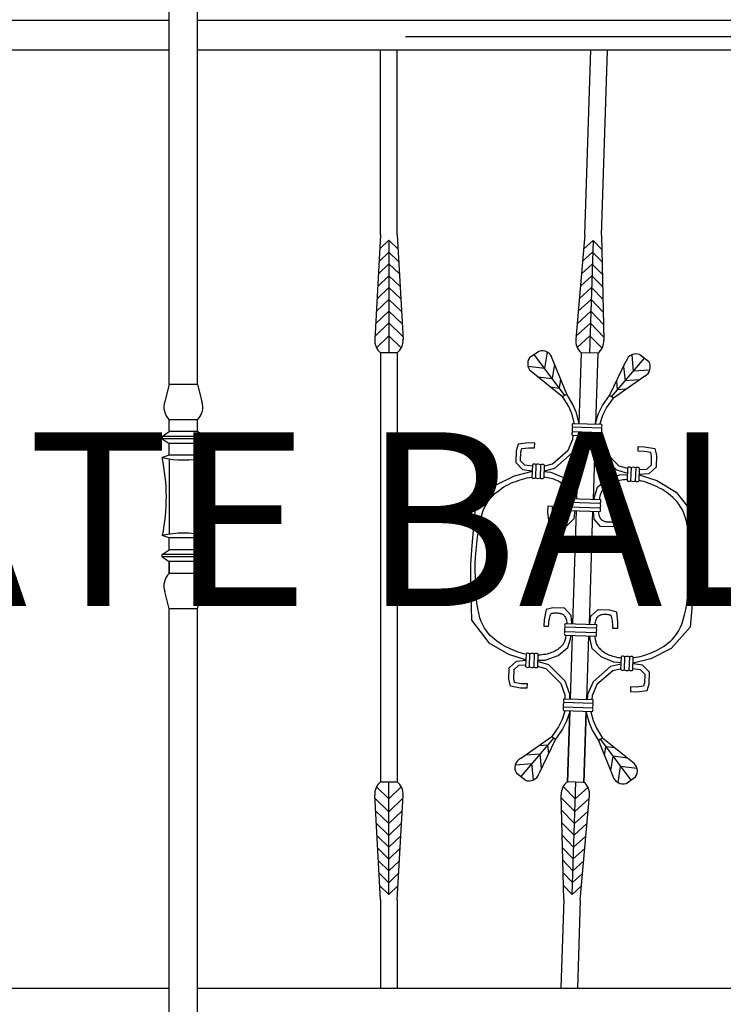
# Model space of a CAD drawing. Units: inches. Extents: x 2278 to 7495, y -71 to 1198.
# Tile 23 of 44: x 5060 to 5084, y 126 to 160. Entities that reach past the tile are written whole.
import ezdxf

# ---------------------------------------------------------------- set-up
doc = ezdxf.new("R2010")
doc.units = ezdxf.units.IN
doc.header["$MEASUREMENT"] = 0
doc.layers.add('A-ANNO-DIMS', color=2, linetype='Continuous', lineweight=18)
doc.layers.add('A-ELEV', color=7, linetype='Continuous', lineweight=25)
doc.styles.get("Standard").update_dxf_attribs({"font": 'arial.ttf'})
doc.dimstyles.get("Standard").update_dxf_attribs({"dimtxt": 6, "dimasz": 3, "dimexe": 0.18, "dimexo": 0.0625, "dimgap": 0.09, "dimtad": 0, "dimtih": 1, "dimtoh": 1, "dimdec": 0, "dimzin": 0, "dimdsep": 46, "dimlunit": 3, "dimtxsty": 'Standard', "dimblk": 'ARCHTICK', "dimcen": 0.09, "dimadec": 0, "dimazin": 0, "dimtfac": 1, "dimtdec": 0, "dimtofl": 0, "dimtmove": 0, "dimatfit": 3, "dimfxl": 1, "dimtolj": 1, "dimtzin": 0, "dimarcsym": 0})

# ---------------------------------------------------------------- blocks, each defined once
blk = doc.blocks.new('BALUSTER-ORNATE-A')
for p, q in [((3.585, 26.003), (3.585, 32.384)), ((4.155, 26.003), (4.155, 32.38)), ((3.585, 26.003), (3.383, 22.393)), ((4.155, 26.003), (4.357, 22.393)), ((3.558, 25.516), (3.87, 25.818)), ((3.87, 25.818), (3.87, 21.929)), ((4.182, 25.516), (3.87, 25.818)), ((3.533, 25.084), (3.87, 25.41)), ((4.207, 25.084), (3.87, 25.41)), ((3.509, 24.653), (3.87, 25.001)), ((4.231, 24.653), (3.87, 25.001)), ((3.485, 24.221), (3.87, 24.593)), ((4.255, 24.221), (3.87, 24.593)), ((3.461, 23.79), (3.87, 24.185)), ((4.279, 23.79), (3.87, 24.185)), ((3.437, 23.358), (3.87, 23.777)), ((4.303, 23.358), (3.87, 23.777)), ((3.413, 22.927), (3.87, 23.369)), ((4.327, 22.927), (3.87, 23.369)), ((3.388, 22.495), (3.87, 22.961)), ((4.352, 22.495), (3.87, 22.961)), ((3.442, 22.106), (3.87, 22.52)), ((4.299, 22.106), (3.87, 22.52)), ((2.128, 21.929), (1.813, 21.699)), ((3.063, 20.442), (1.97, 21.814)), ((2.412, 21.914), (2.339, 21.352)), ((3.585, 21.929), (3.585, 19.485)), ((4.155, 21.929), (3.585, 21.929)), ((4.155, 21.929), (4.155, 19.485)), ((4.677, 20.442), (5.77, 21.814)), ((5.328, 21.914), (5.401, 21.352)), ((5.612, 21.929), (5.927, 21.699)), ((1.774, 21.406), (2.339, 21.352)), ((3.131, 20.487), (2.594, 21.696)), ((2.678, 21.507), (2.613, 21.007)), ((4.609, 20.487), (5.146, 21.696)), ((5.062, 21.507), (5.127, 21.007)), ((5.966, 21.406), (5.401, 21.352)), ((1.936, 21.192), (2.995, 20.398)), ((5.804, 21.192), (4.745, 20.398)), ((2.111, 21.055), (2.613, 21.007)), ((2.907, 20.992), (2.868, 20.688)), ((4.833, 20.992), (4.872, 20.688)), ((5.629, 21.055), (5.127, 21.007)), ((2.562, 20.717), (2.868, 20.688)), ((2.995, 20.398), (3.131, 20.487)), ((3.217, 20.057), (2.995, 20.398)), ((3.36, 20.135), (3.131, 20.487)), ((4.38, 20.135), (4.609, 20.487)), ((4.523, 20.057), (4.745, 20.398)), ((4.745, 20.398), (4.609, 20.487)), ((5.178, 20.717), (4.872, 20.688)), ((3.337, 19.795), (3.217, 20.057)), ((3.49, 19.852), (3.36, 20.135)), ((4.25, 19.852), (4.38, 20.135)), ((4.403, 19.795), (4.523, 20.057)), ((3.421, 19.506), (3.337, 19.795)), ((3.585, 19.526), (3.49, 19.852)), ((4.155, 19.526), (4.25, 19.852)), ((4.319, 19.506), (4.403, 19.795)), ((3.37, 19.485), (4.37, 19.485)), ((3.42, 19.485), (3.421, 19.506)), ((3.583, 19.485), (3.585, 19.526)), ((4.157, 19.485), (4.155, 19.526)), ((4.32, 19.485), (4.319, 19.506)), ((3.37, 19.363), (4.37, 19.363)), ((3.37, 19.2), (4.37, 19.2)), ((3.37, 19.077), (4.37, 19.077)), ((3.396, 18.942), (3.402, 19.077)), ((3.558, 18.908), (3.565, 19.077)), ((3.585, 19.077), (3.585, 16.887)), ((4.155, 19.077), (4.155, 16.887)), ((4.182, 18.908), (4.175, 19.077)), ((4.344, 18.942), (4.338, 19.077)), ((1.513, 18.705), (1.449, 18.469)), ((1.866, 18.759), (1.513, 18.705)), ((2.084, 18.759), (1.866, 18.759)), ((2.084, 18.596), (2.084, 18.759)), ((3.247, 18.557), (3.396, 18.942)), ((3.385, 18.463), (3.558, 18.908)), ((4.355, 18.463), (4.182, 18.908)), ((4.493, 18.557), (4.344, 18.942)), ((5.656, 18.596), (5.656, 18.759)), ((5.656, 18.759), (5.874, 18.759)), ((5.874, 18.759), (6.227, 18.705)), ((6.227, 18.705), (6.291, 18.469)), ((1.449, 18.469), (1.449, 18.069)), ((1.612, 18.447), (1.642, 18.56)), ((1.612, 18.138), (1.612, 18.447)), ((1.642, 18.56), (1.879, 18.596)), ((1.879, 18.596), (2.084, 18.596)), ((2.719, 18.062), (3.247, 18.557)), ((2.801, 17.915), (3.385, 18.463)), ((4.939, 17.915), (4.355, 18.463)), ((5.021, 18.062), (4.493, 18.557)), ((5.861, 18.596), (5.656, 18.596)), ((6.098, 18.56), (5.861, 18.596)), ((6.128, 18.447), (6.098, 18.56)), ((6.128, 18.138), (6.128, 18.447)), ((6.291, 18.469), (6.291, 18.069)), ((1.449, 18.069), (1.694, 17.833)), ((1.767, 17.989), (1.612, 18.138)), ((2.026, 18.021), (2.026, 17.565)), ((2.148, 18.021), (2.148, 17.565)), ((2.311, 18.021), (2.311, 17.565)), ((2.434, 18.021), (2.434, 17.565)), ((2.462, 17.993), (2.719, 18.062)), ((5.278, 17.993), (5.021, 18.062)), ((5.306, 18.021), (5.306, 17.565)), ((5.429, 18.021), (5.429, 17.565)), ((5.592, 18.021), (5.592, 17.565)), ((5.714, 18.021), (5.714, 17.565)), ((5.973, 17.989), (6.128, 18.138)), ((6.291, 18.069), (6.046, 17.833)), ((2.026, 17.782), (1.412, 17.603)), ((1.694, 17.833), (2.026, 17.797)), ((2.026, 17.961), (1.767, 17.989)), ((2.434, 17.99), (2.462, 17.993)), ((2.434, 17.826), (2.492, 17.833)), ((2.683, 17.766), (2.434, 17.777)), ((2.492, 17.833), (2.801, 17.915)), ((3.128, 17.594), (2.683, 17.766)), ((4.612, 17.594), (5.057, 17.766)), ((5.248, 17.833), (4.939, 17.915)), ((5.057, 17.766), (5.306, 17.777)), ((5.306, 17.826), (5.248, 17.833)), ((5.306, 17.99), (5.278, 17.993)), ((5.714, 17.961), (5.973, 17.989)), ((6.046, 17.833), (5.714, 17.797)), ((5.714, 17.782), (6.328, 17.603)), ((1.412, 17.603), (0.722, 17.231)), ((1.23, 17.309), (1.309, 17.35)), ((1.309, 17.35), (1.389, 17.388)), ((1.389, 17.388), (1.469, 17.422)), ((1.469, 17.422), (1.549, 17.454)), ((1.549, 17.454), (1.627, 17.484)), ((1.627, 17.484), (1.705, 17.51)), ((1.705, 17.51), (1.782, 17.533)), ((1.782, 17.533), (1.858, 17.553)), ((1.858, 17.553), (1.933, 17.571)), ((1.933, 17.571), (2.007, 17.585)), ((2.007, 17.585), (2.026, 17.587)), ((2.434, 17.606), (2.499, 17.6)), ((2.499, 17.6), (2.563, 17.592)), ((2.563, 17.592), (2.624, 17.582)), ((2.624, 17.582), (2.683, 17.57)), ((2.683, 17.57), (2.739, 17.556)), ((2.739, 17.556), (2.792, 17.54)), ((2.792, 17.54), (2.843, 17.522)), ((2.843, 17.522), (2.891, 17.503)), ((2.891, 17.503), (2.937, 17.482)), ((2.937, 17.482), (2.981, 17.46)), ((2.981, 17.46), (3.024, 17.436)), ((3.024, 17.436), (3.064, 17.41)), ((3.064, 17.41), (3.102, 17.384)), ((3.102, 17.384), (3.138, 17.357)), ((3.446, 17.313), (3.128, 17.594)), ((3.138, 17.357), (3.171, 17.329)), ((3.171, 17.329), (3.201, 17.301)), ((4.294, 17.313), (4.612, 17.594)), ((4.569, 17.329), (4.539, 17.301)), ((4.602, 17.357), (4.569, 17.329)), ((4.638, 17.384), (4.602, 17.357)), ((4.676, 17.41), (4.638, 17.384)), ((4.716, 17.436), (4.676, 17.41)), ((4.759, 17.46), (4.716, 17.436)), ((4.803, 17.482), (4.759, 17.46)), ((4.849, 17.503), (4.803, 17.482)), ((4.897, 17.522), (4.849, 17.503)), ((4.948, 17.54), (4.897, 17.522)), ((5.001, 17.556), (4.948, 17.54)), ((5.057, 17.57), (5.001, 17.556)), ((5.116, 17.582), (5.057, 17.57)), ((5.177, 17.592), (5.116, 17.582)), ((5.241, 17.6), (5.177, 17.592)), ((5.306, 17.606), (5.241, 17.6)), ((5.733, 17.585), (5.714, 17.587)), ((5.807, 17.571), (5.733, 17.585)), ((5.882, 17.553), (5.807, 17.571)), ((5.958, 17.533), (5.882, 17.553)), ((6.035, 17.51), (5.958, 17.533)), ((6.113, 17.484), (6.035, 17.51)), ((6.191, 17.454), (6.113, 17.484)), ((6.271, 17.422), (6.191, 17.454)), ((6.351, 17.388), (6.271, 17.422)), ((6.328, 17.603), (7.018, 17.231)), ((6.431, 17.35), (6.351, 17.388)), ((6.51, 17.309), (6.431, 17.35)), ((0.722, 17.231), (0.096, 16.469)), ((0.764, 16.975), (0.839, 17.043)), ((0.839, 17.043), (0.916, 17.105)), ((0.916, 17.105), (0.993, 17.163)), ((0.993, 17.163), (1.071, 17.216)), ((1.071, 17.216), (1.15, 17.265)), ((1.15, 17.265), (1.23, 17.309)), ((3.201, 17.301), (3.228, 17.272)), ((3.228, 17.272), (3.252, 17.244)), ((3.252, 17.244), (3.272, 17.217)), ((3.272, 17.217), (3.288, 17.19)), ((3.288, 17.19), (3.303, 17.162)), ((3.303, 17.162), (3.316, 17.134)), ((3.316, 17.134), (3.327, 17.104)), ((3.327, 17.104), (3.337, 17.072)), ((3.337, 17.072), (3.346, 17.038)), ((3.346, 17.038), (3.354, 17.001)), ((3.354, 17.001), (3.361, 16.962)), ((3.528, 17.004), (3.446, 17.313)), ((3.542, 16.887), (3.528, 17.004)), ((4.198, 16.887), (4.212, 17.004)), ((4.212, 17.004), (4.294, 17.313)), ((4.386, 17.001), (4.379, 16.962)), ((4.394, 17.038), (4.386, 17.001)), ((4.403, 17.072), (4.394, 17.038)), ((4.413, 17.104), (4.403, 17.072)), ((4.424, 17.134), (4.413, 17.104)), ((4.437, 17.162), (4.424, 17.134)), ((4.452, 17.19), (4.437, 17.162)), ((4.468, 17.217), (4.452, 17.19)), ((4.489, 17.244), (4.468, 17.217)), ((4.512, 17.272), (4.489, 17.244)), ((4.539, 17.301), (4.512, 17.272)), ((6.59, 17.265), (6.51, 17.309)), ((6.669, 17.216), (6.59, 17.265)), ((6.747, 17.163), (6.669, 17.216)), ((6.824, 17.105), (6.747, 17.163)), ((6.901, 17.043), (6.824, 17.105)), ((6.976, 16.975), (6.901, 17.043)), ((7.018, 17.231), (7.644, 16.469)), ((0.495, 16.624), (0.557, 16.727)), ((0.557, 16.727), (0.623, 16.819)), ((0.623, 16.819), (0.692, 16.9)), ((0.692, 16.9), (0.764, 16.975)), ((3.329, 16.887), (4.411, 16.887)), ((3.329, 16.764), (4.411, 16.764)), ((3.361, 16.962), (3.368, 16.922)), ((3.368, 16.922), (3.374, 16.887)), ((4.372, 16.922), (4.366, 16.887)), ((4.379, 16.962), (4.372, 16.922)), ((7.048, 16.9), (6.976, 16.975)), ((7.117, 16.819), (7.048, 16.9)), ((7.183, 16.727), (7.117, 16.819)), ((7.245, 16.624), (7.183, 16.727)), ((0.096, 16.469), (0.025, 15.162)), ((0.34, 16.227), (0.386, 16.376)), ((0.386, 16.376), (0.438, 16.508)), ((0.438, 16.508), (0.495, 16.624)), ((2.764, 16.599), (2.602, 16.596)), ((2.602, 16.596), (2.602, 16.378)), ((2.602, 16.378), (2.656, 16.024)), ((2.766, 16.522), (2.764, 16.599)), ((2.769, 16.452), (2.766, 16.522)), ((2.775, 16.388), (2.769, 16.452)), ((2.783, 16.331), (2.775, 16.388)), ((2.792, 16.28), (2.783, 16.331)), ((3.329, 16.601), (4.411, 16.601)), ((3.329, 16.479), (4.411, 16.479)), ((3.357, 16.329), (3.346, 16.299)), ((3.368, 16.364), (3.357, 16.329)), ((3.376, 16.401), (3.368, 16.364)), ((3.383, 16.441), (3.376, 16.401)), ((3.388, 16.479), (3.383, 16.441)), ((3.528, 16.206), (3.557, 16.479)), ((3.585, 16.479), (3.585, 12.578)), ((4.155, 16.479), (4.155, 12.578)), ((4.212, 16.206), (4.183, 16.479)), ((4.352, 16.479), (4.357, 16.441)), ((4.357, 16.441), (4.364, 16.401)), ((4.364, 16.401), (4.372, 16.364)), ((4.372, 16.364), (4.383, 16.329)), ((4.383, 16.329), (4.394, 16.299)), ((4.948, 16.28), (4.957, 16.331)), ((4.957, 16.331), (4.965, 16.388)), ((4.965, 16.388), (4.971, 16.452)), ((4.971, 16.452), (4.974, 16.522)), ((4.974, 16.522), (4.976, 16.599)), ((4.976, 16.599), (5.138, 16.596)), ((5.138, 16.378), (5.084, 16.024)), ((5.138, 16.596), (5.138, 16.378)), ((7.302, 16.508), (7.245, 16.624)), ((7.354, 16.376), (7.302, 16.508)), ((7.4, 16.227), (7.354, 16.376)), ((7.644, 16.469), (7.715, 15.162)), ((0.267, 15.87), (0.3, 16.057)), ((0.3, 16.057), (0.34, 16.227)), ((2.656, 16.024), (2.892, 15.961)), ((2.803, 16.237), (2.792, 16.28)), ((2.815, 16.203), (2.803, 16.237)), ((2.825, 16.18), (2.815, 16.203)), ((2.834, 16.166), (2.825, 16.18)), ((2.84, 16.159), (2.834, 16.166)), ((2.846, 16.154), (2.84, 16.159)), ((2.852, 16.151), (2.846, 16.154)), ((2.863, 16.146), (2.852, 16.151)), ((2.88, 16.142), (2.863, 16.146)), ((2.905, 16.137), (2.88, 16.142)), ((2.936, 16.134), (2.905, 16.137)), ((2.971, 16.131), (2.936, 16.134)), ((3.008, 16.129), (2.971, 16.131)), ((3.045, 16.129), (3.008, 16.129)), ((3.081, 16.13), (3.045, 16.129)), ((3.117, 16.133), (3.081, 16.13)), ((3.15, 16.138), (3.117, 16.133)), ((3.179, 16.145), (3.15, 16.138)), ((3.205, 16.154), (3.179, 16.145)), ((3.228, 16.164), (3.205, 16.154)), ((3.249, 16.176), (3.228, 16.164)), ((3.268, 16.19), (3.249, 16.176)), ((3.286, 16.207), (3.268, 16.19)), ((3.303, 16.225), (3.286, 16.207)), ((3.292, 15.961), (3.528, 16.206)), ((3.318, 16.247), (3.303, 16.225)), ((3.333, 16.271), (3.318, 16.247)), ((3.346, 16.299), (3.333, 16.271)), ((4.448, 15.961), (4.212, 16.206)), ((4.394, 16.299), (4.407, 16.271)), ((4.407, 16.271), (4.422, 16.247)), ((4.422, 16.247), (4.437, 16.225)), ((4.437, 16.225), (4.454, 16.207)), ((4.454, 16.207), (4.472, 16.19)), ((4.472, 16.19), (4.491, 16.176)), ((4.491, 16.176), (4.512, 16.164)), ((4.512, 16.164), (4.535, 16.154)), ((4.535, 16.154), (4.561, 16.145)), ((4.561, 16.145), (4.59, 16.138)), ((4.59, 16.138), (4.623, 16.133)), ((4.623, 16.133), (4.659, 16.13)), ((4.659, 16.13), (4.695, 16.129)), ((4.695, 16.129), (4.732, 16.129)), ((4.732, 16.129), (4.769, 16.131)), ((4.769, 16.131), (4.804, 16.134)), ((4.804, 16.134), (4.835, 16.137)), ((4.835, 16.137), (4.86, 16.142)), ((5.084, 16.024), (4.848, 15.961)), ((4.86, 16.142), (4.877, 16.146)), ((4.877, 16.146), (4.888, 16.151)), ((4.888, 16.151), (4.895, 16.154)), ((4.895, 16.154), (4.9, 16.159)), ((4.9, 16.159), (4.906, 16.166)), ((4.906, 16.166), (4.915, 16.18)), ((4.915, 16.18), (4.925, 16.203)), ((4.925, 16.203), (4.937, 16.237)), ((4.937, 16.237), (4.948, 16.28)), ((7.44, 16.057), (7.4, 16.227)), ((7.473, 15.87), (7.44, 16.057)), ((0.217, 15.452), (0.239, 15.667)), ((0.239, 15.667), (0.267, 15.87)), ((2.892, 15.961), (3.292, 15.961)), ((4.848, 15.961), (4.448, 15.961)), ((7.501, 15.667), (7.473, 15.87)), ((7.523, 15.452), (7.501, 15.667)), ((0.199, 15.227), (0.217, 15.452)), ((7.541, 15.227), (7.523, 15.452)), ((0.025, 15.162), (0, 14.529)), ((0.173, 14.759), (0.185, 14.995)), ((0.185, 14.995), (0.199, 15.227)), ((7.555, 14.995), (7.541, 15.227)), ((7.567, 14.759), (7.555, 14.995)), ((7.715, 15.162), (7.74, 14.529)), ((0.163, 14.522), (0.173, 14.759)), ((7.577, 14.522), (7.567, 14.759)), ((0, 14.529), (0.025, 13.895)), ((0.173, 14.298), (0.163, 14.536)), ((0.185, 14.062), (0.173, 14.298)), ((7.555, 14.062), (7.567, 14.298)), ((7.567, 14.298), (7.577, 14.536)), ((7.74, 14.529), (7.715, 13.895)), ((0.199, 13.831), (0.185, 14.062)), ((7.541, 13.831), (7.555, 14.062)), ((0.025, 13.895), (0.096, 12.589)), ((0.217, 13.606), (0.199, 13.831)), ((0.239, 13.391), (0.217, 13.606)), ((7.501, 13.391), (7.523, 13.606)), ((7.523, 13.606), (7.541, 13.831)), ((7.715, 13.895), (7.644, 12.589)), ((0.267, 13.188), (0.239, 13.391)), ((7.473, 13.188), (7.501, 13.391)), ((0.3, 13), (0.267, 13.188)), ((0.34, 12.831), (0.3, 13)), ((2.656, 13.033), (2.602, 12.679)), ((2.892, 13.097), (2.656, 13.033)), ((2.852, 12.907), (2.863, 12.911)), ((2.863, 12.911), (2.88, 12.916)), ((2.88, 12.916), (2.905, 12.92)), ((3.292, 13.097), (2.892, 13.097)), ((2.905, 12.92), (2.936, 12.924)), ((2.936, 12.924), (2.971, 12.927)), ((2.971, 12.927), (3.008, 12.929)), ((3.008, 12.929), (3.045, 12.929)), ((3.045, 12.929), (3.081, 12.928)), ((3.081, 12.928), (3.117, 12.924)), ((3.117, 12.924), (3.15, 12.919)), ((3.15, 12.919), (3.179, 12.912)), ((3.179, 12.912), (3.205, 12.904)), ((3.528, 12.852), (3.292, 13.097)), ((4.212, 12.852), (4.448, 13.097)), ((4.448, 13.097), (4.848, 13.097)), ((4.561, 12.912), (4.535, 12.904)), ((4.59, 12.919), (4.561, 12.912)), ((4.623, 12.924), (4.59, 12.919)), ((4.659, 12.928), (4.623, 12.924)), ((4.695, 12.929), (4.659, 12.928)), ((4.732, 12.929), (4.695, 12.929)), ((4.769, 12.927), (4.732, 12.929)), ((4.804, 12.924), (4.769, 12.927)), ((4.835, 12.92), (4.804, 12.924)), ((4.86, 12.916), (4.835, 12.92)), ((4.848, 13.097), (5.084, 13.033)), ((4.877, 12.911), (4.86, 12.916)), ((4.888, 12.907), (4.877, 12.911)), ((5.084, 13.033), (5.138, 12.679)), ((7.4, 12.831), (7.44, 13)), ((7.44, 13), (7.473, 13.188)), ((0.096, 12.589), (0.722, 11.827)), ((0.386, 12.681), (0.34, 12.831)), ((0.438, 12.549), (0.386, 12.681)), ((2.602, 12.679), (2.602, 12.462)), ((2.766, 12.536), (2.769, 12.605)), ((2.769, 12.605), (2.775, 12.669)), ((2.775, 12.669), (2.783, 12.727)), ((2.783, 12.727), (2.792, 12.778)), ((2.792, 12.778), (2.803, 12.82)), ((2.803, 12.82), (2.815, 12.854)), ((2.815, 12.854), (2.825, 12.878)), ((2.825, 12.878), (2.834, 12.892)), ((2.834, 12.892), (2.84, 12.899)), ((2.84, 12.899), (2.846, 12.903)), ((2.846, 12.903), (2.852, 12.907)), ((3.205, 12.904), (3.228, 12.893)), ((3.228, 12.893), (3.249, 12.881)), ((3.249, 12.881), (3.268, 12.867)), ((3.268, 12.867), (3.286, 12.851)), ((3.286, 12.851), (3.303, 12.832)), ((3.303, 12.832), (3.318, 12.811)), ((3.318, 12.811), (3.333, 12.786)), ((3.329, 12.578), (4.411, 12.578)), ((3.333, 12.786), (3.346, 12.759)), ((3.346, 12.759), (3.357, 12.728)), ((3.357, 12.728), (3.368, 12.694)), ((3.368, 12.694), (3.376, 12.656)), ((3.376, 12.656), (3.383, 12.616)), ((3.383, 12.616), (3.388, 12.578)), ((3.557, 12.578), (3.528, 12.852)), ((4.183, 12.578), (4.212, 12.852)), ((4.357, 12.616), (4.352, 12.578)), ((4.364, 12.656), (4.357, 12.616)), ((4.372, 12.694), (4.364, 12.656)), ((4.383, 12.728), (4.372, 12.694)), ((4.394, 12.759), (4.383, 12.728)), ((4.407, 12.786), (4.394, 12.759)), ((4.422, 12.811), (4.407, 12.786)), ((4.437, 12.832), (4.422, 12.811)), ((4.454, 12.851), (4.437, 12.832)), ((4.472, 12.867), (4.454, 12.851)), ((4.491, 12.881), (4.472, 12.867)), ((4.512, 12.893), (4.491, 12.881)), ((4.535, 12.904), (4.512, 12.893)), ((4.895, 12.903), (4.888, 12.907)), ((4.9, 12.899), (4.895, 12.903)), ((4.906, 12.892), (4.9, 12.899)), ((4.915, 12.878), (4.906, 12.892)), ((4.925, 12.854), (4.915, 12.878)), ((4.937, 12.82), (4.925, 12.854)), ((4.948, 12.778), (4.937, 12.82)), ((4.957, 12.727), (4.948, 12.778)), ((4.965, 12.669), (4.957, 12.727)), ((4.971, 12.605), (4.965, 12.669)), ((4.974, 12.536), (4.971, 12.605)), ((5.138, 12.679), (5.138, 12.462)), ((7.644, 12.589), (7.018, 11.827)), ((7.302, 12.549), (7.354, 12.681)), ((7.354, 12.681), (7.4, 12.831)), ((0.495, 12.433), (0.438, 12.549)), ((0.557, 12.33), (0.495, 12.433)), ((0.623, 12.239), (0.557, 12.33)), ((0.692, 12.157), (0.623, 12.239)), ((2.602, 12.462), (2.764, 12.459)), ((2.764, 12.459), (2.766, 12.536)), ((3.329, 12.456), (4.411, 12.456)), ((3.329, 12.293), (4.411, 12.293)), ((4.976, 12.459), (4.974, 12.536)), ((5.138, 12.462), (4.976, 12.459)), ((7.048, 12.157), (7.117, 12.239)), ((7.117, 12.239), (7.183, 12.33)), ((7.183, 12.33), (7.245, 12.433)), ((7.245, 12.433), (7.302, 12.549)), ((0.764, 12.083), (0.692, 12.157)), ((0.839, 12.015), (0.764, 12.083)), ((0.916, 11.952), (0.839, 12.015)), ((0.993, 11.894), (0.916, 11.952)), ((1.071, 11.841), (0.993, 11.894)), ((3.303, 11.895), (3.288, 11.868)), ((3.316, 11.924), (3.303, 11.895)), ((3.327, 11.954), (3.316, 11.924)), ((3.337, 11.986), (3.327, 11.954)), ((3.329, 12.171), (4.411, 12.171)), ((3.346, 12.02), (3.337, 11.986)), ((3.354, 12.056), (3.346, 12.02)), ((3.361, 12.095), (3.354, 12.056)), ((3.368, 12.136), (3.361, 12.095)), ((3.374, 12.171), (3.368, 12.136)), ((3.446, 11.745), (3.528, 12.053)), ((3.528, 12.053), (3.542, 12.171)), ((3.585, 12.171), (3.585, 9.98)), ((4.155, 12.171), (4.155, 9.98)), ((4.212, 12.053), (4.198, 12.171)), ((4.294, 11.745), (4.212, 12.053)), ((4.366, 12.171), (4.372, 12.136)), ((4.372, 12.136), (4.379, 12.095)), ((4.379, 12.095), (4.386, 12.056)), ((4.386, 12.056), (4.394, 12.02)), ((4.394, 12.02), (4.403, 11.986)), ((4.403, 11.986), (4.413, 11.954)), ((4.413, 11.954), (4.424, 11.924)), ((4.424, 11.924), (4.437, 11.895)), ((4.437, 11.895), (4.452, 11.868)), ((6.669, 11.841), (6.747, 11.894)), ((6.747, 11.894), (6.824, 11.952)), ((6.824, 11.952), (6.901, 12.015)), ((6.901, 12.015), (6.976, 12.083)), ((6.976, 12.083), (7.048, 12.157)), ((0.722, 11.827), (1.412, 11.455)), ((1.15, 11.793), (1.071, 11.841)), ((1.23, 11.748), (1.15, 11.793)), ((1.309, 11.708), (1.23, 11.748)), ((1.389, 11.67), (1.309, 11.708)), ((1.469, 11.635), (1.389, 11.67)), ((1.549, 11.603), (1.469, 11.635)), ((1.627, 11.574), (1.549, 11.603)), ((1.705, 11.548), (1.627, 11.574)), ((2.891, 11.555), (2.843, 11.535)), ((2.937, 11.576), (2.891, 11.555)), ((2.981, 11.598), (2.937, 11.576)), ((3.024, 11.622), (2.981, 11.598)), ((3.064, 11.647), (3.024, 11.622)), ((3.102, 11.673), (3.064, 11.647)), ((3.138, 11.701), (3.102, 11.673)), ((3.128, 11.464), (3.446, 11.745)), ((3.171, 11.729), (3.138, 11.701)), ((3.201, 11.757), (3.171, 11.729)), ((3.228, 11.785), (3.201, 11.757)), ((3.252, 11.813), (3.228, 11.785)), ((3.272, 11.841), (3.252, 11.813)), ((3.288, 11.868), (3.272, 11.841)), ((4.612, 11.464), (4.294, 11.745)), ((4.452, 11.868), (4.468, 11.841)), ((4.468, 11.841), (4.489, 11.813)), ((4.489, 11.813), (4.512, 11.785)), ((4.512, 11.785), (4.539, 11.757)), ((4.539, 11.757), (4.569, 11.729)), ((4.569, 11.729), (4.602, 11.701)), ((4.602, 11.701), (4.638, 11.673)), ((4.638, 11.673), (4.676, 11.647)), ((4.676, 11.647), (4.716, 11.622)), ((4.716, 11.622), (4.759, 11.598)), ((4.759, 11.598), (4.803, 11.576)), ((4.803, 11.576), (4.849, 11.555)), ((4.849, 11.555), (4.897, 11.535)), ((6.035, 11.548), (6.113, 11.574)), ((6.113, 11.574), (6.191, 11.603)), ((6.191, 11.603), (6.271, 11.635)), ((6.271, 11.635), (6.351, 11.67)), ((7.018, 11.827), (6.328, 11.455)), ((6.351, 11.67), (6.431, 11.708)), ((6.431, 11.708), (6.51, 11.748)), ((6.51, 11.748), (6.59, 11.793)), ((6.59, 11.793), (6.669, 11.841)), ((1.412, 11.455), (2.026, 11.276)), ((1.449, 10.988), (1.694, 11.225)), ((1.694, 11.225), (2.026, 11.261)), ((1.782, 11.524), (1.705, 11.548)), ((1.858, 11.504), (1.782, 11.524)), ((1.933, 11.487), (1.858, 11.504)), ((2.007, 11.473), (1.933, 11.487)), ((2.026, 11.47), (2.007, 11.473)), ((2.026, 11.037), (2.026, 11.493)), ((2.148, 11.037), (2.148, 11.493)), ((2.311, 11.037), (2.311, 11.493)), ((2.434, 11.037), (2.434, 11.493)), ((2.499, 11.457), (2.434, 11.451)), ((2.434, 11.28), (2.683, 11.291)), ((2.434, 11.232), (2.492, 11.225)), ((2.492, 11.225), (2.801, 11.143)), ((2.563, 11.465), (2.499, 11.457)), ((2.624, 11.476), (2.563, 11.465)), ((2.683, 11.488), (2.624, 11.476)), ((2.739, 11.502), (2.683, 11.488)), ((2.683, 11.291), (3.128, 11.464)), ((2.792, 11.518), (2.739, 11.502)), ((2.843, 11.535), (2.792, 11.518)), ((5.057, 11.291), (4.612, 11.464)), ((4.897, 11.535), (4.948, 11.518)), ((5.248, 11.225), (4.939, 11.143)), ((4.948, 11.518), (5.001, 11.502)), ((5.001, 11.502), (5.057, 11.488)), ((5.057, 11.488), (5.116, 11.476)), ((5.306, 11.28), (5.057, 11.291)), ((5.116, 11.476), (5.177, 11.465)), ((5.177, 11.465), (5.241, 11.457)), ((5.241, 11.457), (5.306, 11.451)), ((5.306, 11.232), (5.248, 11.225)), ((5.306, 11.037), (5.306, 11.493)), ((5.429, 11.037), (5.429, 11.493)), ((5.592, 11.037), (5.592, 11.493)), ((5.714, 11.037), (5.714, 11.493)), ((5.714, 11.47), (5.733, 11.473)), ((6.328, 11.455), (5.714, 11.276)), ((6.046, 11.225), (5.714, 11.261)), ((5.733, 11.473), (5.807, 11.487)), ((5.807, 11.487), (5.882, 11.504)), ((5.882, 11.504), (5.958, 11.524)), ((5.958, 11.524), (6.035, 11.548)), ((6.291, 10.988), (6.046, 11.225)), ((1.449, 10.589), (1.449, 10.988)), ((1.767, 11.069), (1.612, 10.919)), ((1.612, 10.919), (1.612, 10.611)), ((2.026, 11.097), (1.767, 11.069)), ((2.434, 11.067), (2.462, 11.064)), ((2.462, 11.064), (2.719, 10.996)), ((2.719, 10.996), (3.247, 10.501)), ((2.801, 11.143), (3.385, 10.594)), ((4.939, 11.143), (4.355, 10.594)), ((5.021, 10.996), (4.493, 10.501)), ((5.278, 11.064), (5.021, 10.996)), ((5.306, 11.067), (5.278, 11.064)), ((5.714, 11.097), (5.973, 11.069)), ((5.973, 11.069), (6.128, 10.919)), ((6.128, 10.919), (6.128, 10.611)), ((6.291, 10.589), (6.291, 10.988)), ((1.513, 10.353), (1.449, 10.589)), ((1.612, 10.611), (1.642, 10.498)), ((3.385, 10.594), (3.558, 10.149)), ((4.355, 10.594), (4.182, 10.149)), ((6.128, 10.611), (6.098, 10.498)), ((6.227, 10.353), (6.291, 10.589)), ((1.866, 10.298), (1.513, 10.353)), ((1.642, 10.498), (1.879, 10.461)), ((2.084, 10.298), (1.866, 10.298)), ((1.879, 10.461), (2.084, 10.461)), ((2.084, 10.461), (2.084, 10.298)), ((3.247, 10.501), (3.396, 10.115)), ((4.493, 10.501), (4.344, 10.115)), ((5.861, 10.461), (5.656, 10.461)), ((5.656, 10.461), (5.656, 10.298)), ((5.656, 10.298), (5.874, 10.298)), ((6.098, 10.498), (5.861, 10.461)), ((5.874, 10.298), (6.227, 10.353)), ((3.37, 9.98), (4.37, 9.98)), ((3.37, 9.858), (4.37, 9.858)), ((3.396, 10.115), (3.402, 9.98)), ((3.558, 10.149), (3.565, 9.98)), ((4.182, 10.149), (4.175, 9.98)), ((4.344, 10.115), (4.338, 9.98)), ((3.421, 9.552), (3.337, 9.262)), ((3.37, 9.695), (4.37, 9.695)), ((3.37, 9.573), (4.37, 9.573)), ((3.42, 9.573), (3.421, 9.552)), ((3.585, 9.532), (3.49, 9.205)), ((3.583, 9.573), (3.585, 9.532)), ((3.585, 9.573), (3.585, 7.095)), ((3.585, 7.095), (3.585, 9.573)), ((4.155, 9.573), (4.155, 7.095)), ((4.155, 7.095), (4.155, 9.573)), ((4.157, 9.573), (4.155, 9.532)), ((4.155, 9.532), (4.25, 9.205)), ((4.32, 9.573), (4.319, 9.552)), ((4.319, 9.552), (4.403, 9.262)), ((3.337, 9.262), (3.217, 9.001)), ((3.49, 9.205), (3.36, 8.922)), ((4.25, 9.205), (4.38, 8.922)), ((4.403, 9.262), (4.523, 9.001)), ((3.217, 9.001), (2.995, 8.66)), ((3.36, 8.922), (3.131, 8.571)), ((4.38, 8.922), (4.609, 8.571)), ((4.523, 9.001), (4.745, 8.66)), ((1.936, 7.866), (2.995, 8.66)), ((3.063, 8.615), (1.97, 7.244)), ((3.131, 8.571), (2.594, 7.362)), ((2.995, 8.66), (3.131, 8.571)), ((4.745, 8.66), (4.609, 8.571)), ((4.609, 8.571), (5.146, 7.362)), ((4.677, 8.615), (5.77, 7.244)), ((5.804, 7.866), (4.745, 8.66)), ((2.562, 8.34), (2.868, 8.37)), ((2.907, 8.066), (2.868, 8.37)), ((4.833, 8.066), (4.872, 8.37)), ((5.178, 8.34), (4.872, 8.37)), ((2.111, 8.002), (2.613, 8.051)), ((2.678, 7.551), (2.613, 8.051)), ((5.062, 7.551), (5.127, 8.051)), ((5.629, 8.002), (5.127, 8.051)), ((1.774, 7.651), (2.339, 7.706)), ((2.412, 7.143), (2.339, 7.706)), ((5.328, 7.143), (5.401, 7.706)), ((5.966, 7.651), (5.401, 7.706)), ((2.128, 7.128), (1.813, 7.359)), ((5.612, 7.128), (5.927, 7.359)), ((3.442, 6.952), (3.87, 6.538)), ((3.585, 7.128), (4.155, 7.128)), ((3.87, 3.24), (3.87, 7.128)), ((4.299, 6.952), (3.87, 6.538)), ((3.585, 3.055), (3.383, 6.664)), ((3.388, 6.562), (3.87, 6.097)), ((4.352, 6.562), (3.87, 6.097)), ((4.155, 3.055), (4.357, 6.664)), ((3.413, 6.131), (3.87, 5.689)), ((4.327, 6.131), (3.87, 5.689)), ((3.437, 5.699), (3.87, 5.28)), ((4.303, 5.699), (3.87, 5.28)), ((3.461, 5.268), (3.87, 4.872)), ((4.279, 5.268), (3.87, 4.872)), ((3.485, 4.836), (3.87, 4.464)), ((4.255, 4.836), (3.87, 4.464)), ((3.509, 4.405), (3.87, 4.056)), ((4.231, 4.405), (3.87, 4.056)), ((3.533, 3.973), (3.87, 3.648)), ((4.207, 3.973), (3.87, 3.648)), ((3.558, 3.542), (3.87, 3.24)), ((4.182, 3.542), (3.87, 3.24)), ((3.585, 3.055), (3.585, 0)), ((4.155, 3.055), (4.155, 0))]:
    blk.add_line(p, q)
for centre, radius, start, end in [((3.929, 22.355), 0.547, 176.0178, 231.0717), ((3.811, 22.355), 0.547, 308.9283, 3.9822), ((2.253, 21.595), 0.356, 16.4025, 110.5063), ((5.487, 21.595), 0.356, 69.4937, 163.5975), ((2.111, 21.502), 0.356, 146.575, 240.6788), ((5.629, 21.502), 0.356, 299.3212, 33.425), ((3.475, 19.424), 0.121, 149.7768, 210.2232), ((4.265, 19.424), 0.121, 329.7768, 30.2232), ((3.563, 19.281), 0.209, 157.1017, 202.8983), ((3.475, 19.139), 0.121, 149.7768, 210.2232), ((4.177, 19.281), 0.209, 337.1017, 22.8983), ((4.265, 19.139), 0.121, 329.7768, 30.2232), ((2.087, 17.916), 0.121, 59.7768, 120.2232), ((2.23, 17.828), 0.209, 67.1017, 112.8983), ((2.373, 17.916), 0.121, 59.7768, 120.2232), ((5.368, 17.916), 0.121, 59.7768, 120.2232), ((5.51, 17.828), 0.209, 67.1017, 112.8983), ((5.653, 17.916), 0.121, 59.7768, 120.2232), ((2.087, 17.67), 0.121, 239.7768, 300.2232), ((2.23, 17.758), 0.209, 247.1017, 292.8983), ((2.373, 17.67), 0.121, 239.7768, 300.2232), ((5.368, 17.67), 0.121, 239.7768, 300.2232), ((5.51, 17.758), 0.209, 247.1017, 292.8983), ((5.653, 17.67), 0.121, 239.7768, 300.2232), ((3.434, 16.825), 0.121, 149.7768, 210.2232), ((3.522, 16.683), 0.209, 157.1017, 202.8983), ((4.306, 16.825), 0.121, 329.7768, 30.2232), ((4.218, 16.683), 0.209, 337.1017, 22.8983), ((3.434, 16.54), 0.121, 149.7768, 210.2232), ((4.306, 16.54), 0.121, 329.7768, 30.2232), ((3.434, 12.517), 0.121, 149.7768, 210.2232), ((4.306, 12.517), 0.121, 329.7768, 30.2232), ((3.522, 12.375), 0.209, 157.1017, 202.8983), ((3.434, 12.232), 0.121, 149.7768, 210.2232), ((4.218, 12.375), 0.209, 337.1017, 22.8983), ((4.306, 12.232), 0.121, 329.7768, 30.2232), ((2.087, 11.388), 0.121, 59.7768, 120.2232), ((2.23, 11.3), 0.209, 67.1017, 112.8983), ((2.373, 11.388), 0.121, 59.7768, 120.2232), ((5.368, 11.388), 0.121, 59.7768, 120.2232), ((5.51, 11.3), 0.209, 67.1017, 112.8983), ((5.653, 11.388), 0.121, 59.7768, 120.2232), ((2.087, 11.142), 0.121, 239.7768, 300.2232), ((2.23, 11.23), 0.209, 247.1017, 292.8983), ((2.373, 11.142), 0.121, 239.7768, 300.2232), ((5.368, 11.142), 0.121, 239.7768, 300.2232), ((5.51, 11.23), 0.209, 247.1017, 292.8983), ((5.653, 11.142), 0.121, 239.7768, 300.2232), ((3.475, 9.919), 0.121, 149.7768, 210.2232), ((3.563, 9.776), 0.209, 157.1017, 202.8983), ((4.265, 9.919), 0.121, 329.7768, 30.2232), ((4.177, 9.776), 0.209, 337.1017, 22.8983), ((3.475, 9.634), 0.121, 149.7768, 210.2232), ((4.265, 9.634), 0.121, 329.7768, 30.2232), ((2.111, 7.555), 0.356, 119.3212, 213.425), ((5.629, 7.555), 0.356, 326.575, 60.6788), ((2.253, 7.462), 0.356, 249.4937, 343.5975), ((5.487, 7.462), 0.356, 196.4025, 290.5063), ((3.929, 6.703), 0.547, 128.9283, 183.9822), ((3.811, 6.703), 0.547, 356.0178, 51.0717)]:
    blk.add_arc(centre, radius, start, end)
blk = doc.blocks.new('RAIL-BAR-B')
for p, q in [((17.353, 32.832), (1.059, 32.832)), ((0.203, 26.003), (0.203, 32.38)), ((0.773, 26.003), (0.773, 32.38)), ((0.203, 26.003), (0.001, 22.393)), ((0.773, 26.003), (0.976, 22.393)), ((0.176, 25.516), (0.488, 25.818)), ((0.488, 25.818), (0.488, 21.929)), ((0.801, 25.516), (0.488, 25.818)), ((0.152, 25.084), (0.488, 25.41)), ((0.825, 25.084), (0.488, 25.41)), ((0.128, 24.653), (0.488, 25.001)), ((0.849, 24.653), (0.488, 25.001)), ((0.103, 24.221), (0.488, 24.593)), ((0.873, 24.221), (0.488, 24.593)), ((0.079, 23.79), (0.488, 24.185)), ((0.897, 23.79), (0.488, 24.185)), ((0.055, 23.358), (0.488, 23.777)), ((0.922, 23.358), (0.488, 23.777)), ((0.031, 22.927), (0.488, 23.369)), ((0.946, 22.927), (0.488, 23.369)), ((0.007, 22.495), (0.488, 22.961)), ((0.97, 22.495), (0.488, 22.961)), ((0.06, 22.106), (0.488, 22.52)), ((0.917, 22.106), (0.488, 22.52)), ((0.203, 21.929), (0.203, 7.128)), ((0.773, 21.929), (0.203, 21.929)), ((0.773, 21.929), (0.773, 7.128)), ((0.06, 6.952), (0.488, 6.538)), ((0.203, 7.128), (0.773, 7.128)), ((0.488, 3.24), (0.488, 7.128)), ((0.917, 6.952), (0.488, 6.538)), ((0.203, 3.055), (0.001, 6.664)), ((0.007, 6.562), (0.488, 6.097)), ((0.97, 6.562), (0.488, 6.097)), ((0.773, 3.055), (0.976, 6.664)), ((0.031, 6.131), (0.488, 5.689)), ((0.946, 6.131), (0.488, 5.689)), ((0.055, 5.699), (0.488, 5.28)), ((0.922, 5.699), (0.488, 5.28)), ((0.079, 5.268), (0.488, 4.872)), ((0.897, 5.268), (0.488, 4.872)), ((0.103, 4.836), (0.488, 4.464)), ((0.873, 4.836), (0.488, 4.464)), ((0.128, 4.405), (0.488, 4.056)), ((0.849, 4.405), (0.488, 4.056)), ((0.152, 3.973), (0.488, 3.648)), ((0.825, 3.973), (0.488, 3.648)), ((0.176, 3.542), (0.488, 3.24)), ((0.801, 3.542), (0.488, 3.24)), ((0.203, 3.055), (0.203, 0)), ((0.773, 3.055), (0.773, 0))]:
    blk.add_line(p, q)
for centre, start, end in [((0.547, 22.355), 176.0178, 231.0717), ((0.429, 22.355), 308.9283, 3.9822), ((0.547, 6.703), 128.9283, 183.9822), ((0.429, 6.703), 356.0178, 51.0717)]:
    blk.add_arc(centre, 0.547, start, end)
blk = doc.blocks.new('_ArchTick')
at = {"color": 0, "linetype": 'ByBlock', "const_width": 0.15}
blk.add_lwpolyline([(-0.5, -0.5), (0.5, 0.5)], dxfattribs=at)
blk = doc.blocks.new('*D59')
at = {"layer": 'A-ANNO-DIMS', "color": 0, "lineweight": -2, "transparency": 16777216}
for p, q in [((5096.589, 159.183), (5101.564, 159.183)), ((5101.384, 159.183), (5101.384, 146.185)), ((5101.384, 126.799), (5101.384, 139.796)), ((5096.589, 126.799), (5101.564, 126.799))]:
    blk.add_line(p, q, dxfattribs=at)
at = {"layer": 'Defpoints', "color": 0, "transparency": 16777216}
for p in [(5096.527, 159.183), (5101.384, 159.183), (5096.527, 126.799)]:
    blk.add_point(p, dxfattribs=at)
at = {"layer": 'A-ANNO-DIMS', "color": 0, "lineweight": -2, "transparency": 16777216, "xscale": 3, "yscale": 3, "zscale": 3}
for p, rotation in [((5101.384, 159.183), 90), ((5101.384, 126.799), 270)]:
    blk.add_blockref('_ArchTick', p, dxfattribs=dict(at, rotation=rotation))
at = {"layer": 'A-ANNO-DIMS', "color": 0, "transparency": 16777216, "insert": (5101.384, 142.991), "char_height": 6, "attachment_point": 5}
blk.add_mtext('\\A1;ORNATE BALUSTER 2\'-8 1/2" TYP.', dxfattribs=at)
blk = doc.blocks.new('*D123')
at = {"layer": 'A-ANNO-DIMS', "color": 0, "lineweight": -2, "transparency": 16777216}
for p, q in [((4736.95, 340.157), (4736.95, -23.427)), ((5145.676, -1.81), (5145.676, -23.427)), ((4736.95, -23.247), (4923.929, -23.247)), ((5145.676, -23.247), (4958.697, -23.247))]:
    blk.add_line(p, q, dxfattribs=at)
at = {"layer": 'Defpoints', "color": 0, "transparency": 16777216}
for p in [(4736.95, 340.219), (5145.676, -1.747), (5145.676, -23.247)]:
    blk.add_point(p, dxfattribs=at)
at = {"layer": 'A-ANNO-DIMS', "color": 0, "lineweight": -2, "transparency": 16777216, "xscale": 3, "yscale": 3, "zscale": 3, "rotation": 180}
blk.add_blockref('_ArchTick', (4736.95, -23.247), dxfattribs=at)
at = {"layer": 'A-ANNO-DIMS', "color": 0, "lineweight": -2, "transparency": 16777216, "xscale": 3, "yscale": 3, "zscale": 3}
blk.add_blockref('_ArchTick', (5145.676, -23.247), dxfattribs=at)
at = {"layer": 'A-ANNO-DIMS', "color": 0, "transparency": 16777216, "insert": (4941.313, -23.247), "char_height": 6, "attachment_point": 5}
blk.add_mtext('\\A1;34\'-0 1/2"', dxfattribs=at)
blk = doc.blocks.new('*D130')
at = {"layer": 'A-ANNO-DIMS', "color": 0, "lineweight": -2, "transparency": 16777216}
for p, q in [((5016.176, 99.315), (5016.176, 361.899)), ((5096.176, 99.315), (5096.176, 361.899)), ((5016.176, 361.719), (5048.095, 361.719)), ((5096.176, 361.719), (5064.257, 361.719))]:
    blk.add_line(p, q, dxfattribs=at)
at = {"layer": 'Defpoints', "color": 0, "transparency": 16777216}
for p in [(5096.176, 361.719), (5016.176, 99.253), (5096.176, 99.253)]:
    blk.add_point(p, dxfattribs=at)
at = {"layer": 'A-ANNO-DIMS', "color": 0, "lineweight": -2, "transparency": 16777216, "xscale": 3, "yscale": 3, "zscale": 3, "rotation": 180}
blk.add_blockref('_ArchTick', (5016.176, 361.719), dxfattribs=at)
at = {"layer": 'A-ANNO-DIMS', "color": 0, "lineweight": -2, "transparency": 16777216, "xscale": 3, "yscale": 3, "zscale": 3}
blk.add_blockref('_ArchTick', (5096.176, 361.719), dxfattribs=at)
at = {"layer": 'A-ANNO-DIMS', "color": 0, "transparency": 16777216, "insert": (5056.176, 361.719), "char_height": 6, "attachment_point": 5}
blk.add_mtext('\\A1;6\'-8"', dxfattribs=at)

msp = doc.modelspace()

# ---------------------------------------------------------------- linework, layer by layer
at = {"layer": 'A-ELEV'}
for p, q in [((5065.039, 147.642), (5065.039, 161.577)), ((5066.016, 147.642), (5066.016, 161.577)), ((5065.039, 160.198), (4971.673, 160.198)), ((5145.676, 160.198), (5066.016, 160.198)), ((5065.039, 159.179), (4971.673, 159.179)), ((5145.676, 159.179), (5066.016, 159.179)), ((5065.039, 147.642), (5064.886, 147.049)), ((5066.016, 147.642), (5065.039, 147.642)), ((5066.016, 147.642), (5066.169, 147.049)), ((5066.016, 146.42), (5065.039, 146.42)), ((5065.039, 146.012), (5065.039, 146.42)), ((5066.016, 146.012), (5066.016, 146.42)), ((5064.794, 145.849), (5065.039, 146.012)), ((5064.794, 145.849), (5064.794, 145.768)), ((5066.261, 145.849), (5064.794, 145.849)), ((5064.794, 145.768), (5065.039, 145.605)), ((5066.261, 145.768), (5064.794, 145.768)), ((5066.016, 146.012), (5065.039, 146.012)), ((5066.261, 145.849), (5066.016, 146.012)), ((5066.261, 145.768), (5066.016, 145.605)), ((5066.261, 145.849), (5066.261, 145.768)), ((5066.016, 145.605), (5065.039, 145.605)), ((5065.039, 145.198), (5065.039, 145.605)), ((5066.016, 145.198), (5066.016, 145.605)), ((5065.039, 145.198), (5064.794, 145.116)), ((5066.016, 145.198), (5065.039, 145.198)), ((5065.039, 145.07), (5065.039, 142.474)), ((5066.016, 145.198), (5066.261, 145.116)), ((5066.016, 145.07), (5066.016, 142.474)), ((5065.039, 142.346), (5064.794, 142.428)), ((5066.016, 142.346), (5066.261, 142.428)), ((5065.039, 141.936), (5065.039, 142.346)), ((5066.016, 142.346), (5065.039, 142.346)), ((5066.016, 141.936), (5066.016, 142.346)), ((5064.794, 141.773), (5065.039, 141.936)), ((5064.794, 141.691), (5064.794, 141.773)), ((5066.261, 141.773), (5064.794, 141.773)), ((5064.794, 141.691), (5065.039, 141.529)), ((5066.261, 141.691), (5064.794, 141.691)), ((5066.016, 141.936), (5065.039, 141.936)), ((5066.261, 141.773), (5066.016, 141.936)), ((5066.261, 141.691), (5066.016, 141.529)), ((5066.261, 141.691), (5066.261, 141.773)), ((5065.039, 141.529), (5065.039, 141.121)), ((5065.039, 141.121), (5065.039, 141.529)), ((5066.016, 141.529), (5065.039, 141.529)), ((5066.016, 141.529), (5066.016, 141.121)), ((5066.016, 141.121), (5066.016, 141.529)), ((5066.016, 141.121), (5065.039, 141.121)), ((5065.039, 139.899), (5064.886, 140.492)), ((5066.016, 139.899), (5066.169, 140.492)), ((5066.016, 139.899), (5065.039, 139.899)), ((5065.039, 124.253), (5065.039, 139.899)), ((5066.016, 124.253), (5066.016, 139.899)), ((5065.039, 126.799), (4971.673, 126.799)), ((5145.676, 126.799), (5066.016, 126.799))]:
    msp.add_line(p, q, dxfattribs=at)
for centre, radius, start, end in [((5065.462, 146.856), 0.608, 161.4732, 225.8681), ((5065.593, 146.856), 0.608, 314.1319, 18.5268), ((5065.527, 148.339), 3.305, 257.1818, 282.8182), ((5058.424, 143.743), 6.517, 348.3176, 12.1601), ((5072.631, 143.743), 6.517, 167.8399, 191.6824), ((5065.527, 139.205), 3.305, 77.1818, 102.8182), ((5065.462, 140.685), 0.608, 134.1319, 198.5268), ((5065.593, 140.685), 0.608, 341.4732, 45.8681)]:
    msp.add_arc(centre, radius, start, end, dxfattribs=at)

# ---------------------------------------------------------------- block references
msp.add_blockref('RAIL-BAR-B', (5072.127, 126.799), dxfattribs=at)
at = {"layer": 'A-ELEV', "rotation": 358.17108047433}
msp.add_blockref('BALUSTER-ORNATE-A', (5074.964, 126.93), dxfattribs=at)

# ---------------------------------------------------------------- dimensions: what is measured, and where the dimension line sits
at = {"layer": 'A-ANNO-DIMS'}
for base, p1, p2, picture, middle in [((5096.176, 361.719), (5016.176, 99.253), (5096.176, 99.253), '*D130', (5056.176, 361.719)), ((5145.676, -23.247), (4736.95, 340.219), (5145.676, -1.747), '*D123', (4941.313, -23.247))]:
    dim = msp.add_linear_dim(base=base, p1=p1, p2=p2, dimstyle='Standard', override={"dimdec": 1, "dimlfac": 1, "dimrnd": 0, "dimzin": 1, "dimdsep": 46, "dimlunit": 4, "dimfrac": 2}, dxfattribs=at)
    dim.commit()
    dim.dimension.update_dxf_attribs({"geometry": picture, "text_midpoint": middle})
dim = msp.add_linear_dim(base=(5101.384, 159.183), p1=(5096.527, 126.799), p2=(5096.527, 159.183), angle=90, text='ORNATE BALUSTER <> TYP.', dimstyle='Standard', override={"dimdec": 1, "dimrnd": 0, "dimzin": 1, "dimlunit": 4, "dimfrac": 2}, dxfattribs=at)
dim.commit()
dim.dimension.update_dxf_attribs({"geometry": '*D59', "text_midpoint": (5101.384, 142.991)})

doc.saveas('drawing.dxf')
